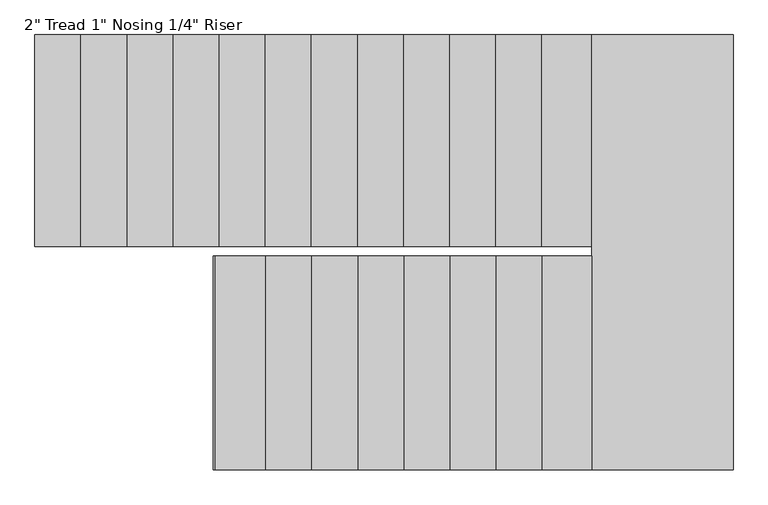
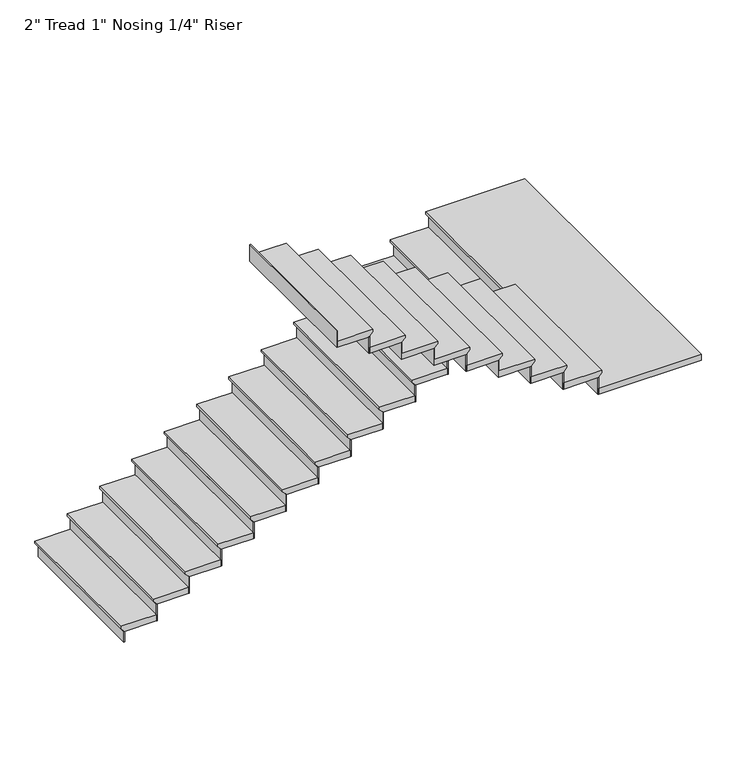
"""IFC4 building model written with IfcOpenShell, lengths in millimetres: stair flight geometry."""

from ifc_helpers import new_model, si_unit, origin, place, context, project, spatial, faceted_brep, source, transform, mapped, element, save


def stair_flight_7472872d(model_context):
    return source(origin(), model_context, "Body", "Brep", [
        faceted_brep([(1811.8890963, 296.3962251, 12311.4954545), (1811.8890963, 296.3962251, 12330.5454545), (1811.8890963, 1464.7962251, 12330.5454545), (1811.8890963, 1464.7962251, 12311.4954545), (1837.2890963, 296.3962251, 12286.0954545), (1837.2890963, 1464.7962251, 12286.0954545), (2091.2890963, 296.3962251, 12330.5454545), (2091.2890963, 1464.7962251, 12330.5454545), (1837.2890963, 1464.7962251, 12279.7454545), (2091.2890963, 1464.7962251, 12279.7454545), (2091.2890963, 296.3962251, 12279.7454545), (1837.2890963, 296.3962251, 12279.7454545)], [[[0, 1, 2, 3]], [[4, 0, 3, 5]], [[2, 1, 6, 7]], [[8, 9, 10, 11]], [[2, 7, 9, 8, 5, 3]], [[8, 11, 4, 5]], [[6, 1, 0, 4, 11, 10]], [[7, 6, 10, 9]]]),
        faceted_brep([(1837.2890963, 296.3962251, 12279.7454545), (1837.2890963, 296.3962251, 12192.0), (1843.6390963, 296.3962251, 12192.0), (1843.6390963, 296.3962251, 12279.7454545), (1837.2890963, 1464.7962251, 12279.7454545), (1843.6390963, 1464.7962251, 12279.7454545), (1843.6390963, 1464.7962251, 12192.0), (1837.2890963, 1464.7962251, 12192.0)], [[[0, 1, 2, 3]], [[4, 5, 6, 7]], [[1, 0, 4, 7]], [[2, 1, 7, 6]], [[3, 2, 6, 5]], [[0, 3, 5, 4]]]),
        faceted_brep([(2091.2890963, 296.3962251, 12418.2909091), (2091.2890963, 296.3962251, 12279.7454545), (2097.6390963, 296.3962251, 12279.7454545), (2097.6390963, 296.3962251, 12418.2909091), (2091.2890963, 1464.7962251, 12418.2909091), (2097.6390963, 1464.7962251, 12418.2909091), (2097.6390963, 1464.7962251, 12279.7454545), (2091.2890963, 1464.7962251, 12279.7454545)], [[[0, 1, 2, 3]], [[4, 5, 6, 7]], [[1, 0, 4, 7]], [[2, 1, 7, 6]], [[3, 2, 6, 5]], [[0, 3, 5, 4]]]),
        faceted_brep([(2065.8890963, 1464.7962251, 12469.0909091), (2065.8890963, 296.3962251, 12469.0909091), (2345.2890963, 296.3962251, 12469.0909091), (2345.2890963, 1464.7962251, 12469.0909091), (2091.2890963, 1464.7962251, 12418.2909091), (2345.2890963, 1464.7962251, 12418.2909091), (2345.2890963, 296.3962251, 12418.2909091), (2091.2890963, 296.3962251, 12418.2909091), (2091.2890963, 1464.7962251, 12424.6409091), (2065.8890963, 1464.7962251, 12450.0409091), (2091.2890963, 296.3962251, 12424.6409091), (2065.8890963, 296.3962251, 12450.0409091)], [[[0, 1, 2, 3]], [[4, 5, 6, 7]], [[0, 3, 5, 4, 8, 9]], [[4, 7, 10, 8]], [[2, 1, 11, 10, 7, 6]], [[3, 2, 6, 5]], [[11, 1, 0, 9]], [[10, 11, 9, 8]]]),
        faceted_brep([(2345.2890963, 296.3962251, 12556.8363636), (2345.2890963, 296.3962251, 12418.2909091), (2351.6390963, 296.3962251, 12418.2909091), (2351.6390963, 296.3962251, 12556.8363636), (2345.2890963, 1464.7962251, 12556.8363636), (2351.6390963, 1464.7962251, 12556.8363636), (2351.6390963, 1464.7962251, 12418.2909091), (2345.2890963, 1464.7962251, 12418.2909091)], [[[0, 1, 2, 3]], [[4, 5, 6, 7]], [[1, 0, 4, 7]], [[2, 1, 7, 6]], [[3, 2, 6, 5]], [[0, 3, 5, 4]]]),
        faceted_brep([(2319.8890963, 1464.7962251, 12607.6363636), (2319.8890963, 296.3962251, 12607.6363636), (2599.2890963, 296.3962251, 12607.6363636), (2599.2890963, 1464.7962251, 12607.6363636), (2345.2890963, 1464.7962251, 12556.8363636), (2599.2890963, 1464.7962251, 12556.8363636), (2599.2890963, 296.3962251, 12556.8363636), (2345.2890963, 296.3962251, 12556.8363636), (2345.2890963, 1464.7962251, 12563.1863636), (2319.8890963, 1464.7962251, 12588.5863636), (2345.2890963, 296.3962251, 12563.1863636), (2319.8890963, 296.3962251, 12588.5863636)], [[[0, 1, 2, 3]], [[4, 5, 6, 7]], [[0, 3, 5, 4, 8, 9]], [[4, 7, 10, 8]], [[2, 1, 11, 10, 7, 6]], [[3, 2, 6, 5]], [[11, 1, 0, 9]], [[10, 11, 9, 8]]]),
        faceted_brep([(2599.2890963, 296.3962251, 12695.3818182), (2599.2890963, 296.3962251, 12556.8363636), (2605.6390963, 296.3962251, 12556.8363636), (2605.6390963, 296.3962251, 12695.3818182), (2599.2890963, 1464.7962251, 12695.3818182), (2605.6390963, 1464.7962251, 12695.3818182), (2605.6390963, 1464.7962251, 12556.8363636), (2599.2890963, 1464.7962251, 12556.8363636)], [[[0, 1, 2, 3]], [[4, 5, 6, 7]], [[1, 0, 4, 7]], [[2, 1, 7, 6]], [[3, 2, 6, 5]], [[0, 3, 5, 4]]]),
        faceted_brep([(2573.8890963, 1464.7962251, 12746.1818182), (2573.8890963, 296.3962251, 12746.1818182), (2853.2890963, 296.3962251, 12746.1818182), (2853.2890963, 1464.7962251, 12746.1818182), (2599.2890963, 1464.7962251, 12695.3818182), (2853.2890963, 1464.7962251, 12695.3818182), (2853.2890963, 296.3962251, 12695.3818182), (2599.2890963, 296.3962251, 12695.3818182), (2599.2890963, 1464.7962251, 12701.7318182), (2573.8890963, 1464.7962251, 12727.1318182), (2599.2890963, 296.3962251, 12701.7318182), (2573.8890963, 296.3962251, 12727.1318182)], [[[0, 1, 2, 3]], [[4, 5, 6, 7]], [[0, 3, 5, 4, 8, 9]], [[4, 7, 10, 8]], [[2, 1, 11, 10, 7, 6]], [[3, 2, 6, 5]], [[11, 1, 0, 9]], [[10, 11, 9, 8]]]),
        faceted_brep([(2853.2890963, 296.3962251, 12833.9272727), (2853.2890963, 296.3962251, 12695.3818182), (2859.6390963, 296.3962251, 12695.3818182), (2859.6390963, 296.3962251, 12833.9272727), (2853.2890963, 1464.7962251, 12833.9272727), (2859.6390963, 1464.7962251, 12833.9272727), (2859.6390963, 1464.7962251, 12695.3818182), (2853.2890963, 1464.7962251, 12695.3818182)], [[[0, 1, 2, 3]], [[4, 5, 6, 7]], [[1, 0, 4, 7]], [[2, 1, 7, 6]], [[3, 2, 6, 5]], [[0, 3, 5, 4]]]),
        faceted_brep([(2827.8890963, 1464.7962251, 12884.7272727), (2827.8890963, 296.3962251, 12884.7272727), (3107.2890963, 296.3962251, 12884.7272727), (3107.2890963, 1464.7962251, 12884.7272727), (2853.2890963, 1464.7962251, 12833.9272727), (3107.2890963, 1464.7962251, 12833.9272727), (3107.2890963, 296.3962251, 12833.9272727), (2853.2890963, 296.3962251, 12833.9272727), (2853.2890963, 1464.7962251, 12840.2772727), (2827.8890963, 1464.7962251, 12865.6772727), (2853.2890963, 296.3962251, 12840.2772727), (2827.8890963, 296.3962251, 12865.6772727)], [[[0, 1, 2, 3]], [[4, 5, 6, 7]], [[0, 3, 5, 4, 8, 9]], [[4, 7, 10, 8]], [[2, 1, 11, 10, 7, 6]], [[3, 2, 6, 5]], [[11, 1, 0, 9]], [[10, 11, 9, 8]]]),
        faceted_brep([(3107.2890963, 296.3962251, 12972.4727273), (3107.2890963, 296.3962251, 12833.9272727), (3113.6390963, 296.3962251, 12833.9272727), (3113.6390963, 296.3962251, 12972.4727273), (3107.2890963, 1464.7962251, 12972.4727273), (3113.6390963, 1464.7962251, 12972.4727273), (3113.6390963, 1464.7962251, 12833.9272727), (3107.2890963, 1464.7962251, 12833.9272727)], [[[0, 1, 2, 3]], [[4, 5, 6, 7]], [[1, 0, 4, 7]], [[2, 1, 7, 6]], [[3, 2, 6, 5]], [[0, 3, 5, 4]]]),
        faceted_brep([(3081.8890963, 1464.7962251, 13023.2727273), (3081.8890963, 296.3962251, 13023.2727273), (3361.2890963, 296.3962251, 13023.2727273), (3361.2890963, 1464.7962251, 13023.2727273), (3107.2890963, 1464.7962251, 12972.4727273), (3361.2890963, 1464.7962251, 12972.4727273), (3361.2890963, 296.3962251, 12972.4727273), (3107.2890963, 296.3962251, 12972.4727273), (3107.2890963, 1464.7962251, 12978.8227273), (3081.8890963, 1464.7962251, 13004.2227273), (3107.2890963, 296.3962251, 12978.8227273), (3081.8890963, 296.3962251, 13004.2227273)], [[[0, 1, 2, 3]], [[4, 5, 6, 7]], [[0, 3, 5, 4, 8, 9]], [[4, 7, 10, 8]], [[2, 1, 11, 10, 7, 6]], [[3, 2, 6, 5]], [[11, 1, 0, 9]], [[10, 11, 9, 8]]]),
        faceted_brep([(3361.2890963, 296.3962251, 13111.0181818), (3361.2890963, 296.3962251, 12972.4727273), (3367.6390963, 296.3962251, 12972.4727273), (3367.6390963, 296.3962251, 13111.0181818), (3361.2890963, 1464.7962251, 13111.0181818), (3367.6390963, 1464.7962251, 13111.0181818), (3367.6390963, 1464.7962251, 12972.4727273), (3361.2890963, 1464.7962251, 12972.4727273)], [[[0, 1, 2, 3]], [[4, 5, 6, 7]], [[1, 0, 4, 7]], [[2, 1, 7, 6]], [[3, 2, 6, 5]], [[0, 3, 5, 4]]]),
        faceted_brep([(3335.8890963, 1464.7962251, 13161.8181818), (3335.8890963, 296.3962251, 13161.8181818), (3615.2890963, 296.3962251, 13161.8181818), (3615.2890963, 1464.7962251, 13161.8181818), (3361.2890963, 1464.7962251, 13111.0181818), (3615.2890963, 1464.7962251, 13111.0181818), (3615.2890963, 296.3962251, 13111.0181818), (3361.2890963, 296.3962251, 13111.0181818), (3361.2890963, 1464.7962251, 13117.3681818), (3335.8890963, 1464.7962251, 13142.7681818), (3361.2890963, 296.3962251, 13117.3681818), (3335.8890963, 296.3962251, 13142.7681818)], [[[0, 1, 2, 3]], [[4, 5, 6, 7]], [[0, 3, 5, 4, 8, 9]], [[4, 7, 10, 8]], [[2, 1, 11, 10, 7, 6]], [[3, 2, 6, 5]], [[11, 1, 0, 9]], [[10, 11, 9, 8]]]),
        faceted_brep([(3615.2890963, 296.3962251, 13249.5636364), (3615.2890963, 296.3962251, 13111.0181818), (3621.6390963, 296.3962251, 13111.0181818), (3621.6390963, 296.3962251, 13249.5636364), (3615.2890963, 1464.7962251, 13249.5636364), (3621.6390963, 1464.7962251, 13249.5636364), (3621.6390963, 1464.7962251, 13111.0181818), (3615.2890963, 1464.7962251, 13111.0181818)], [[[0, 1, 2, 3]], [[4, 5, 6, 7]], [[1, 0, 4, 7]], [[2, 1, 7, 6]], [[3, 2, 6, 5]], [[0, 3, 5, 4]]]),
        faceted_brep([(3589.8890963, 1464.7962251, 13300.3636364), (3589.8890963, 296.3962251, 13300.3636364), (3869.2890963, 296.3962251, 13300.3636364), (3869.2890963, 1464.7962251, 13300.3636364), (3615.2890963, 1464.7962251, 13249.5636364), (3869.2890963, 1464.7962251, 13249.5636364), (3869.2890963, 296.3962251, 13249.5636364), (3615.2890963, 296.3962251, 13249.5636364), (3615.2890963, 1464.7962251, 13255.9136364), (3589.8890963, 1464.7962251, 13281.3136364), (3615.2890963, 296.3962251, 13255.9136364), (3589.8890963, 296.3962251, 13281.3136364)], [[[0, 1, 2, 3]], [[4, 5, 6, 7]], [[0, 3, 5, 4, 8, 9]], [[4, 7, 10, 8]], [[2, 1, 11, 10, 7, 6]], [[3, 2, 6, 5]], [[11, 1, 0, 9]], [[10, 11, 9, 8]]]),
        faceted_brep([(3869.2890963, 296.3962251, 13388.1090909), (3869.2890963, 296.3962251, 13249.5636364), (3875.6390963, 296.3962251, 13249.5636364), (3875.6390963, 296.3962251, 13388.1090909), (3869.2890963, 1464.7962251, 13388.1090909), (3875.6390963, 1464.7962251, 13388.1090909), (3875.6390963, 1464.7962251, 13249.5636364), (3869.2890963, 1464.7962251, 13249.5636364)], [[[0, 1, 2, 3]], [[4, 5, 6, 7]], [[1, 0, 4, 7]], [[2, 1, 7, 6]], [[3, 2, 6, 5]], [[0, 3, 5, 4]]]),
        faceted_brep([(3843.8890963, 1464.7962251, 13438.9090909), (3843.8890963, 296.3962251, 13438.9090909), (4123.2890963, 296.3962251, 13438.9090909), (4123.2890963, 1464.7962251, 13438.9090909), (3869.2890963, 1464.7962251, 13388.1090909), (4123.2890963, 1464.7962251, 13388.1090909), (4123.2890963, 296.3962251, 13388.1090909), (3869.2890963, 296.3962251, 13388.1090909), (3869.2890963, 1464.7962251, 13394.4590909), (3843.8890963, 1464.7962251, 13419.8590909), (3869.2890963, 296.3962251, 13394.4590909), (3843.8890963, 296.3962251, 13419.8590909)], [[[0, 1, 2, 3]], [[4, 5, 6, 7]], [[0, 3, 5, 4, 8, 9]], [[4, 7, 10, 8]], [[2, 1, 11, 10, 7, 6]], [[3, 2, 6, 5]], [[11, 1, 0, 9]], [[10, 11, 9, 8]]]),
        faceted_brep([(4123.2890963, 296.3962251, 13526.6545455), (4123.2890963, 296.3962251, 13388.1090909), (4129.6390963, 296.3962251, 13388.1090909), (4129.6390963, 296.3962251, 13526.6545455), (4123.2890963, 1464.7962251, 13526.6545455), (4129.6390963, 1464.7962251, 13526.6545455), (4129.6390963, 1464.7962251, 13388.1090909), (4123.2890963, 1464.7962251, 13388.1090909)], [[[0, 1, 2, 3]], [[4, 5, 6, 7]], [[1, 0, 4, 7]], [[2, 1, 7, 6]], [[3, 2, 6, 5]], [[0, 3, 5, 4]]]),
        faceted_brep([(4097.8890963, 1464.7962251, 13577.4545455), (4097.8890963, 296.3962251, 13577.4545455), (4377.2890963, 296.3962251, 13577.4545455), (4377.2890963, 1464.7962251, 13577.4545455), (4123.2890963, 1464.7962251, 13526.6545455), (4377.2890963, 1464.7962251, 13526.6545455), (4377.2890963, 296.3962251, 13526.6545455), (4123.2890963, 296.3962251, 13526.6545455), (4123.2890963, 1464.7962251, 13533.0045455), (4097.8890963, 1464.7962251, 13558.4045455), (4123.2890963, 296.3962251, 13533.0045455), (4097.8890963, 296.3962251, 13558.4045455)], [[[0, 1, 2, 3]], [[4, 5, 6, 7]], [[0, 3, 5, 4, 8, 9]], [[4, 7, 10, 8]], [[2, 1, 11, 10, 7, 6]], [[3, 2, 6, 5]], [[11, 1, 0, 9]], [[10, 11, 9, 8]]]),
        faceted_brep([(4377.2890963, 296.3962251, 13665.2), (4377.2890963, 296.3962251, 13526.6545455), (4383.6390963, 296.3962251, 13526.6545455), (4383.6390963, 296.3962251, 13665.2), (4377.2890963, 1464.7962251, 13665.2), (4383.6390963, 1464.7962251, 13665.2), (4383.6390963, 1464.7962251, 13526.6545455), (4377.2890963, 1464.7962251, 13526.6545455)], [[[0, 1, 2, 3]], [[4, 5, 6, 7]], [[1, 0, 4, 7]], [[2, 1, 7, 6]], [[3, 2, 6, 5]], [[0, 3, 5, 4]]]),
        faceted_brep([(4351.8890963, 1464.7962251, 13716.0), (4351.8890963, 296.3962251, 13716.0), (4631.2890963, 296.3962251, 13716.0), (4631.2890963, 1464.7962251, 13716.0), (4377.2890963, 1464.7962251, 13665.2), (4631.2890963, 1464.7962251, 13665.2), (4631.2890963, 296.3962251, 13665.2), (4377.2890963, 296.3962251, 13665.2), (4377.2890963, 1464.7962251, 13671.55), (4351.8890963, 1464.7962251, 13696.95), (4377.2890963, 296.3962251, 13671.55), (4351.8890963, 296.3962251, 13696.95)], [[[0, 1, 2, 3]], [[4, 5, 6, 7]], [[0, 3, 5, 4, 8, 9]], [[4, 7, 10, 8]], [[2, 1, 11, 10, 7, 6]], [[3, 2, 6, 5]], [[11, 1, 0, 9]], [[10, 11, 9, 8]]]),
        faceted_brep([(4631.2890963, 296.3962251, 13803.7454545), (4631.2890963, 296.3962251, 13665.2), (4637.6390963, 296.3962251, 13665.2), (4637.6390963, 296.3962251, 13803.7454545), (4631.2890963, 1464.7962251, 13803.7454545), (4637.6390963, 1464.7962251, 13803.7454545), (4637.6390963, 1464.7962251, 13665.2), (4631.2890963, 1464.7962251, 13665.2)], [[[0, 1, 2, 3]], [[4, 5, 6, 7]], [[1, 0, 4, 7]], [[2, 1, 7, 6]], [[3, 2, 6, 5]], [[0, 3, 5, 4]]]),
        faceted_brep([(4605.8890963, 1464.7962251, 13854.5454545), (4605.8890963, 296.3962251, 13854.5454545), (4906.4326586, 296.3962251, 13854.5454545), (4906.4326586, 1464.7962251, 13854.5454545), (4631.2890963, 1464.7962251, 13803.7454545), (4906.4326586, 1464.7962251, 13803.7454545), (4906.4326586, 296.3962251, 13803.7454545), (4631.2890963, 296.3962251, 13803.7454545), (4631.2890963, 1464.7962251, 13810.0954545), (4605.8890963, 1464.7962251, 13835.4954545), (4631.2890963, 296.3962251, 13810.0954545), (4605.8890963, 296.3962251, 13835.4954545)], [[[0, 1, 2, 3]], [[4, 5, 6, 7]], [[0, 3, 5, 4, 8, 9]], [[4, 7, 10, 8]], [[2, 1, 11, 10, 7, 6]], [[3, 2, 6, 5]], [[11, 1, 0, 9]], [[10, 11, 9, 8]]]),
        faceted_brep([(4906.4326586, 296.3962251, 13942.2909091), (4906.4326586, 296.3962251, 13803.7454545), (4912.7826586, 296.3962251, 13803.7454545), (4912.7826586, 296.3962251, 13942.2909091), (4906.4326586, 1464.7962251, 13942.2909091), (4912.7826586, 1464.7962251, 13942.2909091), (4912.7826586, 1464.7962251, 13803.7454545), (4906.4326586, 1464.7962251, 13803.7454545)], [[[0, 1, 2, 3]], [[4, 5, 6, 7]], [[1, 0, 4, 7]], [[2, 1, 7, 6]], [[3, 2, 6, 5]], [[0, 3, 5, 4]]]),
        faceted_brep([(4855.6326586, -935.5037749, 13993.0909091), (5659.9890963, -935.5037749, 13993.0909091), (5659.9890963, 1464.7962251, 13993.0909091), (4881.0326586, 1464.7962251, 13993.0909091), (4881.0326586, 245.5962251, 13993.0909091), (4855.6326586, 245.5962251, 13993.0909091), (5659.9890963, -935.5037749, 13942.2909091), (4855.6326586, -935.5037749, 13942.2909091), (4855.6326586, 245.5962251, 13942.2909091), (4881.0326586, 245.5962251, 13942.2909091), (4881.0326586, 296.3962251, 13942.2909091), (4906.4326586, 296.3962251, 13942.2909091), (4906.4326586, 1464.7962251, 13942.2909091), (5659.9890963, 1464.7962251, 13942.2909091), (4906.4326586, 1464.7962251, 13948.6409091), (4881.0326586, 1464.7962251, 13974.0409091), (4906.4326586, 296.3962251, 13948.6409091), (4881.0326586, 296.3962251, 13974.0409091)], [[[0, 1, 2, 3, 4, 5]], [[6, 7, 8, 9, 10, 11, 12, 13]], [[1, 0, 7, 6]], [[2, 1, 6, 13]], [[3, 2, 13, 12, 14, 15]], [[12, 11, 16, 14]], [[11, 10, 17, 16]], [[4, 3, 15, 17, 10, 9]], [[5, 4, 9, 8]], [[0, 5, 8, 7]], [[15, 14, 16, 17]]]),
        faceted_brep([(4855.6326586, 245.5962251, 14080.8363636), (4855.6326586, 245.5962251, 13942.2909091), (4849.2826586, 245.5962251, 13942.2909091), (4849.2826586, 245.5962251, 14080.8363636), (4855.6326586, -935.5037749, 14080.8363636), (4849.2826586, -935.5037749, 14080.8363636), (4849.2826586, -935.5037749, 13942.2909091), (4855.6326586, -935.5037749, 13942.2909091)], [[[0, 1, 2, 3]], [[4, 5, 6, 7]], [[1, 0, 4, 7]], [[2, 1, 7, 6]], [[3, 2, 6, 5]], [[0, 3, 5, 4]]]),
        faceted_brep([(4881.0326586, -935.5037749, 14131.6363636), (4881.0326586, 245.5962251, 14131.6363636), (4580.4890963, 245.5962251, 14131.6363636), (4580.4890963, -935.5037749, 14131.6363636), (4855.6326586, -935.5037749, 14080.8363636), (4580.4890963, -935.5037749, 14080.8363636), (4580.4890963, 245.5962251, 14080.8363636), (4855.6326586, 245.5962251, 14080.8363636), (4855.6326586, -935.5037749, 14087.1863636), (4881.0326586, -935.5037749, 14112.5863636), (4855.6326586, 245.5962251, 14087.1863636), (4881.0326586, 245.5962251, 14112.5863636)], [[[0, 1, 2, 3]], [[4, 5, 6, 7]], [[0, 3, 5, 4, 8, 9]], [[4, 7, 10, 8]], [[2, 1, 11, 10, 7, 6]], [[3, 2, 6, 5]], [[11, 1, 0, 9]], [[10, 11, 9, 8]]]),
        faceted_brep([(4580.4890963, 245.5962251, 14219.3818182), (4580.4890963, 245.5962251, 14080.8363636), (4574.1390963, 245.5962251, 14080.8363636), (4574.1390963, 245.5962251, 14219.3818182), (4580.4890963, -935.5037749, 14219.3818182), (4574.1390963, -935.5037749, 14219.3818182), (4574.1390963, -935.5037749, 14080.8363636), (4580.4890963, -935.5037749, 14080.8363636)], [[[0, 1, 2, 3]], [[4, 5, 6, 7]], [[1, 0, 4, 7]], [[2, 1, 7, 6]], [[3, 2, 6, 5]], [[0, 3, 5, 4]]]),
        faceted_brep([(4605.8890963, -935.5037749, 14270.1818182), (4605.8890963, 245.5962251, 14270.1818182), (4326.4890963, 245.5962251, 14270.1818182), (4326.4890963, -935.5037749, 14270.1818182), (4580.4890963, -935.5037749, 14219.3818182), (4326.4890963, -935.5037749, 14219.3818182), (4326.4890963, 245.5962251, 14219.3818182), (4580.4890963, 245.5962251, 14219.3818182), (4580.4890963, -935.5037749, 14225.7318182), (4605.8890963, -935.5037749, 14251.1318182), (4580.4890963, 245.5962251, 14225.7318182), (4605.8890963, 245.5962251, 14251.1318182)], [[[0, 1, 2, 3]], [[4, 5, 6, 7]], [[0, 3, 5, 4, 8, 9]], [[4, 7, 10, 8]], [[2, 1, 11, 10, 7, 6]], [[3, 2, 6, 5]], [[11, 1, 0, 9]], [[10, 11, 9, 8]]]),
        faceted_brep([(4326.4890963, 245.5962251, 14357.9272727), (4326.4890963, 245.5962251, 14219.3818182), (4320.1390963, 245.5962251, 14219.3818182), (4320.1390963, 245.5962251, 14357.9272727), (4326.4890963, -935.5037749, 14357.9272727), (4320.1390963, -935.5037749, 14357.9272727), (4320.1390963, -935.5037749, 14219.3818182), (4326.4890963, -935.5037749, 14219.3818182)], [[[0, 1, 2, 3]], [[4, 5, 6, 7]], [[1, 0, 4, 7]], [[2, 1, 7, 6]], [[3, 2, 6, 5]], [[0, 3, 5, 4]]]),
        faceted_brep([(4351.8890963, -935.5037749, 14408.7272727), (4351.8890963, 245.5962251, 14408.7272727), (4072.4890963, 245.5962251, 14408.7272727), (4072.4890963, -935.5037749, 14408.7272727), (4326.4890963, -935.5037749, 14357.9272727), (4072.4890963, -935.5037749, 14357.9272727), (4072.4890963, 245.5962251, 14357.9272727), (4326.4890963, 245.5962251, 14357.9272727), (4326.4890963, -935.5037749, 14364.2772727), (4351.8890963, -935.5037749, 14389.6772727), (4326.4890963, 245.5962251, 14364.2772727), (4351.8890963, 245.5962251, 14389.6772727)], [[[0, 1, 2, 3]], [[4, 5, 6, 7]], [[0, 3, 5, 4, 8, 9]], [[4, 7, 10, 8]], [[2, 1, 11, 10, 7, 6]], [[3, 2, 6, 5]], [[11, 1, 0, 9]], [[10, 11, 9, 8]]]),
        faceted_brep([(4072.4890963, 245.5962251, 14496.4727273), (4072.4890963, 245.5962251, 14357.9272727), (4066.1390963, 245.5962251, 14357.9272727), (4066.1390963, 245.5962251, 14496.4727273), (4072.4890963, -935.5037749, 14496.4727273), (4066.1390963, -935.5037749, 14496.4727273), (4066.1390963, -935.5037749, 14357.9272727), (4072.4890963, -935.5037749, 14357.9272727)], [[[0, 1, 2, 3]], [[4, 5, 6, 7]], [[1, 0, 4, 7]], [[2, 1, 7, 6]], [[3, 2, 6, 5]], [[0, 3, 5, 4]]]),
        faceted_brep([(4097.8890963, -935.5037749, 14547.2727273), (4097.8890963, 245.5962251, 14547.2727273), (3818.4890963, 245.5962251, 14547.2727273), (3818.4890963, -935.5037749, 14547.2727273), (4072.4890963, -935.5037749, 14496.4727273), (3818.4890963, -935.5037749, 14496.4727273), (3818.4890963, 245.5962251, 14496.4727273), (4072.4890963, 245.5962251, 14496.4727273), (4072.4890963, -935.5037749, 14502.8227273), (4097.8890963, -935.5037749, 14528.2227273), (4072.4890963, 245.5962251, 14502.8227273), (4097.8890963, 245.5962251, 14528.2227273)], [[[0, 1, 2, 3]], [[4, 5, 6, 7]], [[0, 3, 5, 4, 8, 9]], [[4, 7, 10, 8]], [[2, 1, 11, 10, 7, 6]], [[3, 2, 6, 5]], [[11, 1, 0, 9]], [[10, 11, 9, 8]]]),
        faceted_brep([(3818.4890963, 245.5962251, 14635.0181818), (3818.4890963, 245.5962251, 14496.4727273), (3812.1390963, 245.5962251, 14496.4727273), (3812.1390963, 245.5962251, 14635.0181818), (3818.4890963, -935.5037749, 14635.0181818), (3812.1390963, -935.5037749, 14635.0181818), (3812.1390963, -935.5037749, 14496.4727273), (3818.4890963, -935.5037749, 14496.4727273)], [[[0, 1, 2, 3]], [[4, 5, 6, 7]], [[1, 0, 4, 7]], [[2, 1, 7, 6]], [[3, 2, 6, 5]], [[0, 3, 5, 4]]]),
        faceted_brep([(3843.8890963, -935.5037749, 14685.8181818), (3843.8890963, 245.5962251, 14685.8181818), (3564.4890963, 245.5962251, 14685.8181818), (3564.4890963, -935.5037749, 14685.8181818), (3818.4890963, -935.5037749, 14635.0181818), (3564.4890963, -935.5037749, 14635.0181818), (3564.4890963, 245.5962251, 14635.0181818), (3818.4890963, 245.5962251, 14635.0181818), (3818.4890963, -935.5037749, 14641.3681818), (3843.8890963, -935.5037749, 14666.7681818), (3818.4890963, 245.5962251, 14641.3681818), (3843.8890963, 245.5962251, 14666.7681818)], [[[0, 1, 2, 3]], [[4, 5, 6, 7]], [[0, 3, 5, 4, 8, 9]], [[4, 7, 10, 8]], [[2, 1, 11, 10, 7, 6]], [[3, 2, 6, 5]], [[11, 1, 0, 9]], [[10, 11, 9, 8]]]),
        faceted_brep([(3564.4890963, 245.5962251, 14773.5636364), (3564.4890963, 245.5962251, 14635.0181818), (3558.1390963, 245.5962251, 14635.0181818), (3558.1390963, 245.5962251, 14773.5636364), (3564.4890963, -935.5037749, 14773.5636364), (3558.1390963, -935.5037749, 14773.5636364), (3558.1390963, -935.5037749, 14635.0181818), (3564.4890963, -935.5037749, 14635.0181818)], [[[0, 1, 2, 3]], [[4, 5, 6, 7]], [[1, 0, 4, 7]], [[2, 1, 7, 6]], [[3, 2, 6, 5]], [[0, 3, 5, 4]]]),
        faceted_brep([(3589.8890963, -935.5037749, 14824.3636364), (3589.8890963, 245.5962251, 14824.3636364), (3310.4890963, 245.5962251, 14824.3636364), (3310.4890963, -935.5037749, 14824.3636364), (3564.4890963, -935.5037749, 14773.5636364), (3310.4890963, -935.5037749, 14773.5636364), (3310.4890963, 245.5962251, 14773.5636364), (3564.4890963, 245.5962251, 14773.5636364), (3564.4890963, -935.5037749, 14779.9136364), (3589.8890963, -935.5037749, 14805.3136364), (3564.4890963, 245.5962251, 14779.9136364), (3589.8890963, 245.5962251, 14805.3136364)], [[[0, 1, 2, 3]], [[4, 5, 6, 7]], [[0, 3, 5, 4, 8, 9]], [[4, 7, 10, 8]], [[2, 1, 11, 10, 7, 6]], [[3, 2, 6, 5]], [[11, 1, 0, 9]], [[10, 11, 9, 8]]]),
        faceted_brep([(3310.4890963, 245.5962251, 14912.1090909), (3310.4890963, 245.5962251, 14773.5636364), (3304.1390963, 245.5962251, 14773.5636364), (3304.1390963, 245.5962251, 14912.1090909), (3310.4890963, -935.5037749, 14912.1090909), (3304.1390963, -935.5037749, 14912.1090909), (3304.1390963, -935.5037749, 14773.5636364), (3310.4890963, -935.5037749, 14773.5636364)], [[[0, 1, 2, 3]], [[4, 5, 6, 7]], [[1, 0, 4, 7]], [[2, 1, 7, 6]], [[3, 2, 6, 5]], [[0, 3, 5, 4]]]),
        faceted_brep([(3335.8890963, -935.5037749, 14962.9090909), (3335.8890963, 245.5962251, 14962.9090909), (3056.4890963, 245.5962251, 14962.9090909), (3056.4890963, -935.5037749, 14962.9090909), (3310.4890963, -935.5037749, 14912.1090909), (3056.4890963, -935.5037749, 14912.1090909), (3056.4890963, 245.5962251, 14912.1090909), (3310.4890963, 245.5962251, 14912.1090909), (3310.4890963, -935.5037749, 14918.4590909), (3335.8890963, -935.5037749, 14943.8590909), (3310.4890963, 245.5962251, 14918.4590909), (3335.8890963, 245.5962251, 14943.8590909)], [[[0, 1, 2, 3]], [[4, 5, 6, 7]], [[0, 3, 5, 4, 8, 9]], [[4, 7, 10, 8]], [[2, 1, 11, 10, 7, 6]], [[3, 2, 6, 5]], [[11, 1, 0, 9]], [[10, 11, 9, 8]]]),
        faceted_brep([(3056.4890963, 245.5962251, 15050.6545455), (3056.4890963, 245.5962251, 14912.1090909), (3050.1390963, 245.5962251, 14912.1090909), (3050.1390963, 245.5962251, 15050.6545455), (3056.4890963, -935.5037749, 15050.6545455), (3050.1390963, -935.5037749, 15050.6545455), (3050.1390963, -935.5037749, 14912.1090909), (3056.4890963, -935.5037749, 14912.1090909)], [[[0, 1, 2, 3]], [[4, 5, 6, 7]], [[1, 0, 4, 7]], [[2, 1, 7, 6]], [[3, 2, 6, 5]], [[0, 3, 5, 4]]]),
        faceted_brep([(2802.4890963, 245.5962251, 15189.2), (2802.4890963, 245.5962251, 15050.6545455), (2796.1390963, 245.5962251, 15050.6545455), (2796.1390963, 245.5962251, 15189.2), (2802.4890963, -935.5037749, 15189.2), (2796.1390963, -935.5037749, 15189.2), (2796.1390963, -935.5037749, 15050.6545455), (2802.4890963, -935.5037749, 15050.6545455)], [[[0, 1, 2, 3]], [[4, 5, 6, 7]], [[1, 0, 4, 7]], [[2, 1, 7, 6]], [[3, 2, 6, 5]], [[0, 3, 5, 4]]]),
        faceted_brep([(3081.8890963, -935.5037749, 15101.4545455), (3081.8890963, 245.5962251, 15101.4545455), (2802.4890963, 245.5962251, 15101.4545455), (2802.4890963, -935.5037749, 15101.4545455), (3056.4890963, -935.5037749, 15050.6545455), (2802.4890963, -935.5037749, 15050.6545455), (2802.4890963, 245.5962251, 15050.6545455), (3056.4890963, 245.5962251, 15050.6545455), (3056.4890963, -935.5037749, 15057.0045455), (3081.8890963, -935.5037749, 15082.4045455), (3056.4890963, 245.5962251, 15057.0045455), (3081.8890963, 245.5962251, 15082.4045455)], [[[0, 1, 2, 3]], [[4, 5, 6, 7]], [[0, 3, 5, 4, 8, 9]], [[4, 7, 10, 8]], [[2, 1, 11, 10, 7, 6]], [[3, 2, 6, 5]], [[11, 1, 0, 9]], [[10, 11, 9, 8]]]),
    ])


if __name__ == "__main__":
    model = new_model("IFC4")
    model_context = context("Model", 3, world=origin())
    ifc_project = project(units=[si_unit("LENGTHUNIT", "METRE", prefix="MILLI")], contexts=[model_context])
    site = spatial("IfcSite", under=ifc_project)
    building = spatial("IfcBuilding", under=site)
    placement = place(None, origin())
    stair_flight_shape = stair_flight_7472872d(model_context)
    element("IfcStairFlight", 1, ObjectType="2\" Tread 1\" Nosing 1/4\" Riser", at=placement, inside=building, context=model_context, shape_type="MappedRepresentation", body=[
        mapped(stair_flight_shape, transform((0.0, 0.0, 0.0), x_axis=(1.0, 0.0, 0.0), y_axis=(0.0, 1.0, 0.0), z_axis=(0.0, 0.0, 1.0))),
    ])
    save(model, "model.ifc")
